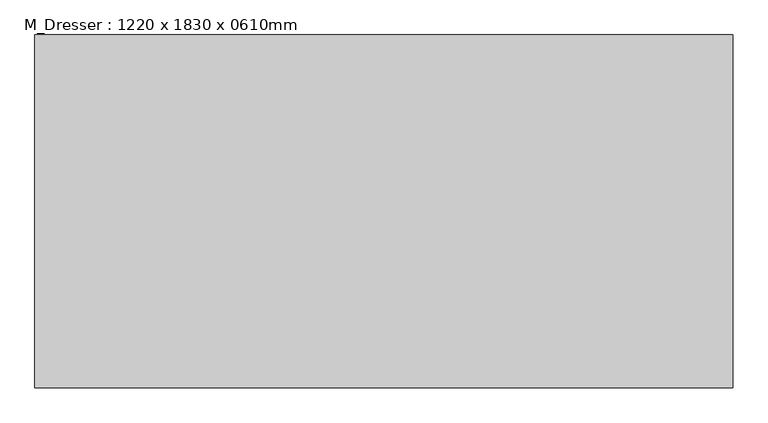
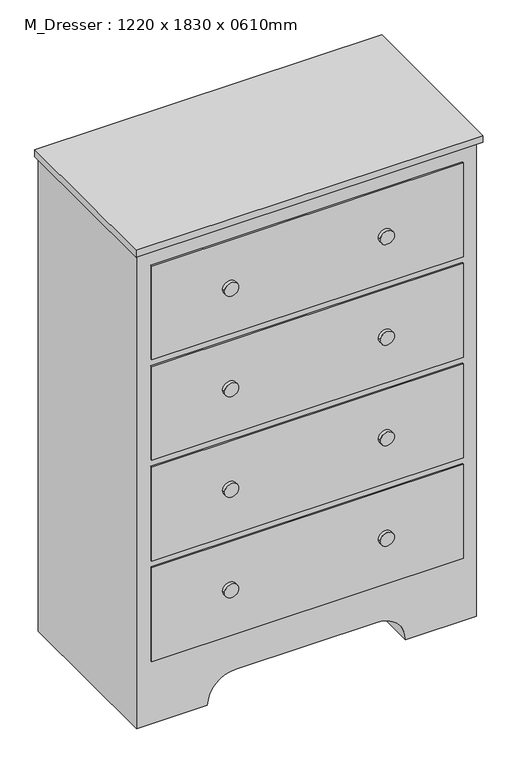
"""IFC4 building model written with IfcOpenShell, lengths in millimetres: furniture geometry, M_Dresser : 1220 x 1830 x 0610mm."""

from ifc_helpers import new_model, si_unit, point, frame, frame_2d, origin, place, context, project, spatial, polyline, circle_curve, trimmed, segment, composite_curve, outline, extrude, source, transform, mapped, element, save


def m_dresser_1220_x_1830_x_0610mm_7cb11019(model_context):
    return source(origin(), model_context, "Body", "SweptSolid", [
        extrude(outline(polyline([(353.5067402, -58.1629541), (353.5067402, -687.2129541), (-891.8932598, -687.2129541), (-891.8932598, -58.1629541), (353.5067402, -58.1629541)])), frame((0.0, 0.0, 1804.6), z_axis=(0.0, 0.0, 1.0), x_axis=(1.0, 0.0, 0.0)), (0.0, 0.0, 1.0), 25.4),
        extrude(outline(composite_curve([segment(polyline([(0.0, 340.8067402), (1804.6, 340.8067402), (1804.6, -879.1932598), (0.0, -879.1932598), (0.0, -625.1932598)]), True, "CONTINUOUS"), segment(trimmed(circle_curve(frame_2d((0.0, -523.5932598)), 101.6), [point((0.0, -625.1932598))], [point((101.6, -523.5932598))], True, "CARTESIAN"), True, "CONTINUOUS"), segment(polyline([(101.6, -523.5932598), (101.6, -14.7932598)]), True, "CONTINUOUS"), segment(trimmed(circle_curve(frame_2d((0.0, -14.7932598)), 101.6), [point((101.6, -14.7932598))], [point((0.0, 86.8067402))], True, "CARTESIAN"), True, "CONTINUOUS"), segment(polyline([(0.0, 86.8067402), (0.0, 340.8067402)]), True, "CONTINUOUS")], self_intersect=False)), frame((0.0, -668.1629541, 0.0), z_axis=(0.0, 1.0, 0.0), x_axis=(0.0, 0.0, 1.0)), (0.0, 0.0, 1.0), 610.0),
        extrude(outline(composite_curve([segment(trimmed(circle_curve(frame_2d((1563.15, 10.4067402)), 25.4), [point((1563.15, -14.9932598))], [point((1563.15, 35.8067402))], False, "CARTESIAN"), True, "CONTINUOUS"), segment(trimmed(circle_curve(frame_2d((1563.15, 10.4067402)), 25.4), [point((1563.15, 35.8067402))], [point((1563.15, -14.9932598))], False, "CARTESIAN"), True, "CONTINUOUS")], self_intersect=False)), frame((0.0, -687.2129541, 0.0), z_axis=(0.0, 1.0, 0.0), x_axis=(0.0, 0.0, 1.0)), (0.0, 0.0, 1.0), 12.7),
        extrude(outline(composite_curve([segment(trimmed(circle_curve(frame_2d((1181.85, 10.4067402)), 25.4), [point((1181.85, -14.9932598))], [point((1181.85, 35.8067402))], False, "CARTESIAN"), True, "CONTINUOUS"), segment(trimmed(circle_curve(frame_2d((1181.85, 10.4067402)), 25.4), [point((1181.85, 35.8067402))], [point((1181.85, -14.9932598))], False, "CARTESIAN"), True, "CONTINUOUS")], self_intersect=False)), frame((0.0, -687.2129541, 0.0), z_axis=(0.0, 1.0, 0.0), x_axis=(0.0, 0.0, 1.0)), (0.0, 0.0, 1.0), 12.7),
        extrude(outline(composite_curve([segment(trimmed(circle_curve(frame_2d((800.55, 10.4067402)), 25.4), [point((800.55, -14.9932598))], [point((800.55, 35.8067402))], False, "CARTESIAN"), True, "CONTINUOUS"), segment(trimmed(circle_curve(frame_2d((800.55, 10.4067402)), 25.4), [point((800.55, 35.8067402))], [point((800.55, -14.9932598))], False, "CARTESIAN"), True, "CONTINUOUS")], self_intersect=False)), frame((0.0, -687.2129541, 0.0), z_axis=(0.0, 1.0, 0.0), x_axis=(0.0, 0.0, 1.0)), (0.0, 0.0, 1.0), 12.7),
        extrude(outline(composite_curve([segment(trimmed(circle_curve(frame_2d((419.25, 10.4067402)), 25.4), [point((419.25, -14.9932598))], [point((419.25, 35.8067402))], False, "CARTESIAN"), True, "CONTINUOUS"), segment(trimmed(circle_curve(frame_2d((419.25, 10.4067402)), 25.4), [point((419.25, 35.8067402))], [point((419.25, -14.9932598))], False, "CARTESIAN"), True, "CONTINUOUS")], self_intersect=False)), frame((0.0, -687.2129541, 0.0), z_axis=(0.0, 1.0, 0.0), x_axis=(0.0, 0.0, 1.0)), (0.0, 0.0, 1.0), 12.7),
        extrude(outline(composite_curve([segment(trimmed(circle_curve(frame_2d((419.25, -548.7932598)), 25.4), [point((419.25, -574.1932598))], [point((419.25, -523.3932598))], False, "CARTESIAN"), True, "CONTINUOUS"), segment(trimmed(circle_curve(frame_2d((419.25, -548.7932598)), 25.4), [point((419.25, -523.3932598))], [point((419.25, -574.1932598))], False, "CARTESIAN"), True, "CONTINUOUS")], self_intersect=False)), frame((0.0, -687.2129541, 0.0), z_axis=(0.0, 1.0, 0.0), x_axis=(0.0, 0.0, 1.0)), (0.0, 0.0, 1.0), 12.7),
        extrude(outline(composite_curve([segment(trimmed(circle_curve(frame_2d((800.55, -548.7932598)), 25.4), [point((800.55, -574.1932598))], [point((800.55, -523.3932598))], False, "CARTESIAN"), True, "CONTINUOUS"), segment(trimmed(circle_curve(frame_2d((800.55, -548.7932598)), 25.4), [point((800.55, -523.3932598))], [point((800.55, -574.1932598))], False, "CARTESIAN"), True, "CONTINUOUS")], self_intersect=False)), frame((0.0, -687.2129541, 0.0), z_axis=(0.0, 1.0, 0.0), x_axis=(0.0, 0.0, 1.0)), (0.0, 0.0, 1.0), 12.7),
        extrude(outline(composite_curve([segment(trimmed(circle_curve(frame_2d((1181.85, -548.7932598)), 25.4), [point((1181.85, -574.1932598))], [point((1181.85, -523.3932598))], False, "CARTESIAN"), True, "CONTINUOUS"), segment(trimmed(circle_curve(frame_2d((1181.85, -548.7932598)), 25.4), [point((1181.85, -523.3932598))], [point((1181.85, -574.1932598))], False, "CARTESIAN"), True, "CONTINUOUS")], self_intersect=False)), frame((0.0, -687.2129541, 0.0), z_axis=(0.0, 1.0, 0.0), x_axis=(0.0, 0.0, 1.0)), (0.0, 0.0, 1.0), 12.7),
        extrude(outline(composite_curve([segment(trimmed(circle_curve(frame_2d((1563.15, -548.7932598)), 25.4), [point((1563.15, -574.1932598))], [point((1563.15, -523.3932598))], False, "CARTESIAN"), True, "CONTINUOUS"), segment(trimmed(circle_curve(frame_2d((1563.15, -548.7932598)), 25.4), [point((1563.15, -523.3932598))], [point((1563.15, -574.1932598))], False, "CARTESIAN"), True, "CONTINUOUS")], self_intersect=False)), frame((0.0, -687.2129541, 0.0), z_axis=(0.0, 1.0, 0.0), x_axis=(0.0, 0.0, 1.0)), (0.0, 0.0, 1.0), 12.7),
        extrude(outline(polyline([(290.0067402, -674.5129541), (-828.3932598, -674.5129541), (-828.3932598, -668.1629541), (290.0067402, -668.1629541), (290.0067402, -674.5129541)])), frame((0.0, 0.0, 1385.2), z_axis=(0.0, 0.0, 1.0), x_axis=(1.0, 0.0, 0.0)), (0.0, 0.0, 1.0), 355.9),
        extrude(outline(polyline([(290.0067402, -674.5129541), (-828.3932598, -674.5129541), (-828.3932598, -668.1629541), (290.0067402, -668.1629541), (290.0067402, -674.5129541)])), frame((0.0, 0.0, 1003.9), z_axis=(0.0, 0.0, 1.0), x_axis=(1.0, 0.0, 0.0)), (0.0, 0.0, 1.0), 355.9),
        extrude(outline(polyline([(290.0067402, -674.5129541), (-828.3932598, -674.5129541), (-828.3932598, -668.1629541), (290.0067402, -668.1629541), (290.0067402, -674.5129541)])), frame((0.0, 0.0, 622.6), z_axis=(0.0, 0.0, 1.0), x_axis=(1.0, 0.0, 0.0)), (0.0, 0.0, 1.0), 355.9),
        extrude(outline(polyline([(290.0067402, -674.5129541), (-828.3932598, -674.5129541), (-828.3932598, -668.1629541), (290.0067402, -668.1629541), (290.0067402, -674.5129541)])), frame((0.0, 0.0, 241.3), z_axis=(0.0, 0.0, 1.0), x_axis=(1.0, 0.0, 0.0)), (0.0, 0.0, 1.0), 355.9),
    ])


if __name__ == "__main__":
    model = new_model("IFC4")
    model_context = context("Model", 3, world=origin())
    ifc_project = project(units=[si_unit("LENGTHUNIT", "METRE", prefix="MILLI")], contexts=[model_context])
    site = spatial("IfcSite", under=ifc_project)
    building = spatial("IfcBuilding", under=site)
    placement = place(None, origin())
    m_dresser_1220_x_1830_x_0610mm_shape = m_dresser_1220_x_1830_x_0610mm_7cb11019(model_context)
    element("IfcFurniture", 1, ObjectType="M_Dresser : 1220 x 1830 x 0610mm", at=placement, inside=building, context=model_context, shape_type="MappedRepresentation", body=[
        mapped(m_dresser_1220_x_1830_x_0610mm_shape, transform((0.0, 0.0, 0.0), x_axis=(1.0, 0.0, 0.0), y_axis=(0.0, 1.0, 0.0), z_axis=(0.0, 0.0, 1.0))),
    ])
    save(model, "model.ifc")

# Revit data of these elements
# Type "M_Dresser : 1220 x 1830 x 0610mm"
#   Depth = 2' - 0.01575"
#   Height = 6' - 0.04724"
#   Width = 4' - 0.0315"
#   Dresser Material = Laminate - Ivory, Glossy
#   Drawer Material = Laminate, Ivory, Matte
#   Knob Material = Cherry
#   Default Elevation = 0
# Element 1 (IfcFurniture, "M_Dresser : 1220 x 1830 x 0610mm")
#   Materials on its faces: "Laminate, Ivory, Matte", "Cherry", "Laminate - Ivory, Glossy"
# Materials
#   "Laminate - Ivory, Glossy": colour RGB 247 247 239, transparency 0
#   "Laminate, Ivory, Matte": class "Plastic", colour RGB 247 247 239, transparency 0, Description = "Plastic Laminate - Ivory, Matte", Cost = 0
#   "Cherry": class "Wood", colour RGB 226 177 128, transparency 0, Description = "Prunus Serotina", Cost = 0
